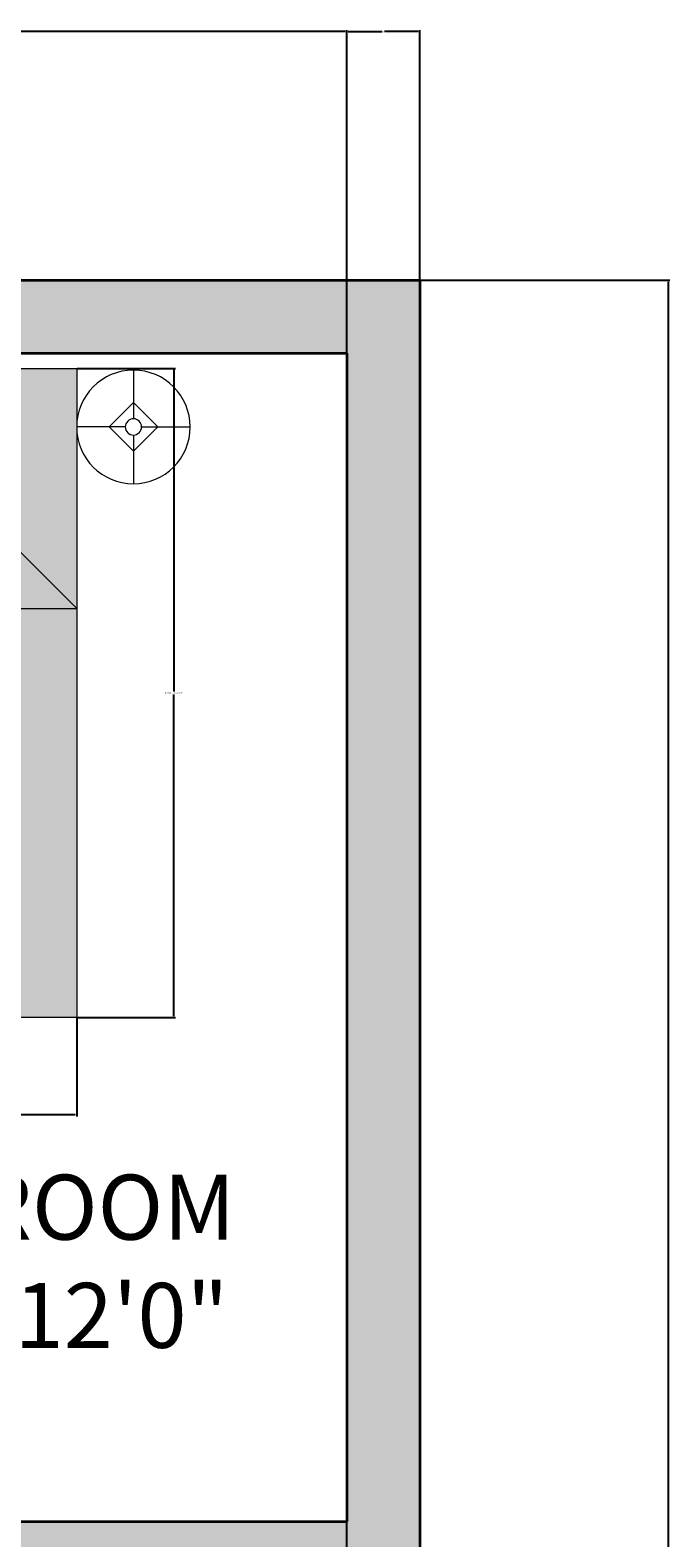
# Model space of a CAD drawing. Units: inches. Extents: x 1567 to 1964, y 1813 to 2447.
# Tile 28 of 28: x 1885 to 1964, y 2261 to 2447. Entities that reach past the tile are written whole.
import ezdxf

# ---------------------------------------------------------------- set-up
doc = ezdxf.new("R2010")
doc.units = ezdxf.units.IN
for name, color, linetype, lineweight in [('A-ANNO-DIMS', 2, 'Continuous', 18), ('A-AREA-IDEN', 7, 'Continuous', 18), ('A-FURN', 8, 'Continuous', 18), ('A-WALL', 7, 'Continuous', 35)]:
    doc.layers.add(name, color=color, linetype=linetype, lineweight=lineweight)
doc.layers.add('A-FURN-PATT', color=252, linetype='Continuous', lineweight=13, true_color=0x939598)
doc.layers.add('A-WALL-PATT', color=251, linetype='Continuous', lineweight=13, true_color=0x636466)
doc.styles.get("Standard").update_dxf_attribs({"font": 'arial.ttf'})
doc.dimstyles.get("Standard").update_dxf_attribs({"dimtxt": 0.18, "dimasz": 0.18, "dimexe": 0.18, "dimexo": 0.0625, "dimgap": 0.09, "dimtad": 0, "dimtih": 1, "dimtoh": 1, "dimdec": 4, "dimzin": 0, "dimdsep": 46, "dimtxsty": 'Standard', "dimcen": 0.09, "dimadec": 0, "dimazin": 0, "dimtfac": 1, "dimtdec": 4, "dimtofl": 0, "dimtmove": 0, "dimatfit": 3, "dimfxl": 1, "dimtolj": 1, "dimtzin": 0, "dimarcsym": 0})

# ---------------------------------------------------------------- blocks, each defined once
blk = doc.blocks.new('Bed - Queen')
for p, q in [((0, -80.00003), (0, 0)), ((0, 0), (59.99999, 0)), ((59.99999, 0), (59.99999, -80.00003)), ((7.99999, -1.2), (28.79998, -1.2)), ((7.99999, -14.4), (7.99999, -1.2)), ((28.79998, -1.2), (28.79998, -14.4)), ((31.19999, -1.2), (51.99999, -1.2)), ((31.19999, -14.4), (31.19999, -1.2)), ((51.99999, -1.2), (51.99999, -16.4)), ((0, -14.4), (44.8, -14.4)), ((59.99999, -29.6), (44.8, -14.4)), ((44.8, -14.4), (44.8, -29.6)), ((51.99999, -16.4), (46.79936, -16.4)), ((44.8, -16.8), (0, -16.8)), ((44.8, -29.6), (59.99999, -29.6)), ((59.99999, -80.00003), (0, -80.00003))]:
    blk.add_line(p, q)
blk = doc.blocks.new('Lamp - Table')
for p, q in [((0, 7), (0, 1)), ((0, 3), (-3, 0)), ((3, 0), (0, 3)), ((-1, 0), (-7, 0)), ((-3, 0), (0, -3)), ((0, -3), (3, 0)), ((1, 0), (7, 0)), ((0, -1), (0, -7))]:
    blk.add_line(p, q)
for radius in [7, 1]:
    blk.add_circle((0, 0), radius)
blk = doc.blocks.new('*D15')
at = {"layer": 'A-ANNO-DIMS', "color": 0, "lineweight": -2, "transparency": 16777216}
for p, q in [((1891.17, 2405.42), (1903.29, 2405.42)), ((1903.11, 2405.24), (1903.11, 2365.61)), ((1903.11, 2325.6), (1903.11, 2365.23)), ((1891.17, 2325.42), (1903.29, 2325.42))]:
    blk.add_line(p, q, dxfattribs=at)
at = {"layer": 'A-ANNO-DIMS', "color": 0, "transparency": 16777216}
for points in [[(1903.08, 2405.24), (1903.14, 2405.24), (1903.11, 2405.42)], [(1903.08, 2325.6), (1903.14, 2325.6), (1903.11, 2325.42)]]:
    blk.add_solid(points, dxfattribs=at)
at = {"layer": 'Defpoints', "color": 0, "transparency": 16777216}
for p in [(1891.11, 2405.42), (1903.11, 2405.42), (1891.11, 2325.42)]:
    blk.add_point(p, dxfattribs=at)
at = {"layer": 'A-ANNO-DIMS', "color": 0, "transparency": 16777216, "insert": (1903.11, 2365.42), "char_height": 0.18, "attachment_point": 5}
blk.add_mtext('\\A1;QUEEN BED 80 TYP.', dxfattribs=at)
blk = doc.blocks.new('*D16')
at = {"layer": 'A-ANNO-DIMS', "color": 0, "lineweight": -2, "transparency": 16777216}
for p, q in [((1831.11, 2325.36), (1831.11, 2313.24)), ((1891.11, 2325.36), (1891.11, 2313.24)), ((1831.29, 2313.42), (1860.58, 2313.42)), ((1890.93, 2313.42), (1861.64, 2313.42))]:
    blk.add_line(p, q, dxfattribs=at)
at = {"layer": 'A-ANNO-DIMS', "color": 0, "transparency": 16777216}
for points in [[(1831.29, 2313.45), (1831.29, 2313.39), (1831.11, 2313.42)], [(1890.93, 2313.45), (1890.93, 2313.39), (1891.11, 2313.42)]]:
    blk.add_solid(points, dxfattribs=at)
at = {"layer": 'Defpoints', "color": 0, "transparency": 16777216}
for p in [(1831.11, 2325.42), (1891.11, 2325.42), (1891.11, 2313.42)]:
    blk.add_point(p, dxfattribs=at)
at = {"layer": 'A-ANNO-DIMS', "color": 0, "transparency": 16777216, "insert": (1861.11, 2313.42), "char_height": 0.18, "attachment_point": 5}
blk.add_mtext('\\A1;60 TYP.', dxfattribs=at)
blk = doc.blocks.new('*D40')
at = {"layer": 'A-ANNO-DIMS', "color": 0, "lineweight": -2, "transparency": 16777216}
for p, q in [((1933.49, 2416.29), (1964.26, 2416.29)), ((1964.08, 2416.11), (1964.08, 2130.47)), ((1964.08, 1844.47), (1964.08, 2130.11)), ((1933.49, 1844.29), (1964.26, 1844.29))]:
    blk.add_line(p, q, dxfattribs=at)
at = {"layer": 'A-ANNO-DIMS', "color": 0, "transparency": 16777216}
for points in [[(1964.05, 2416.11), (1964.11, 2416.11), (1964.08, 2416.29)], [(1964.05, 1844.47), (1964.11, 1844.47), (1964.08, 1844.29)]]:
    blk.add_solid(points, dxfattribs=at)
at = {"layer": 'Defpoints', "color": 0, "transparency": 16777216}
for p in [(1933.43, 2416.29), (1964.08, 2416.29), (1933.43, 1844.29)]:
    blk.add_point(p, dxfattribs=at)
at = {"layer": 'A-ANNO-DIMS', "color": 0, "transparency": 16777216, "insert": (1964.08, 2130.29), "char_height": 0.18, "attachment_point": 5}
blk.add_mtext('\\A1;572', dxfattribs=at)
blk = doc.blocks.new('*D46')
at = {"layer": 'A-ANNO-DIMS', "color": 0, "lineweight": -2, "transparency": 16777216}
for p, q in [((1924.43, 2407.35), (1924.43, 2447.12)), ((1924.61, 2446.94), (1928.78, 2446.94)), ((1933.25, 2446.94), (1929.08, 2446.94)), ((1933.43, 2416.35), (1933.43, 2447.12))]:
    blk.add_line(p, q, dxfattribs=at)
at = {"layer": 'A-ANNO-DIMS', "color": 0, "transparency": 16777216}
for points in [[(1924.61, 2446.97), (1924.61, 2446.91), (1924.43, 2446.94)], [(1933.25, 2446.97), (1933.25, 2446.91), (1933.43, 2446.94)]]:
    blk.add_solid(points, dxfattribs=at)
at = {"layer": 'Defpoints', "color": 0, "transparency": 16777216}
for p in [(1924.43, 2446.94), (1933.43, 2416.29), (1924.43, 2407.29)]:
    blk.add_point(p, dxfattribs=at)
at = {"layer": 'A-ANNO-DIMS', "color": 0, "transparency": 16777216, "insert": (1928.93, 2446.94), "char_height": 0.18, "attachment_point": 5}
blk.add_mtext('\\A1;9', dxfattribs=at)
blk = doc.blocks.new('*D71')
at = {"layer": 'A-ANNO-DIMS', "color": 0, "lineweight": -2, "transparency": 16777216}
for p, q in [((1799.43, 1910.75), (1799.43, 2447.12)), ((1799.61, 2446.94), (1861.65, 2446.94)), ((1924.25, 2446.94), (1862.21, 2446.94)), ((1924.43, 1910.75), (1924.43, 2447.12))]:
    blk.add_line(p, q, dxfattribs=at)
at = {"layer": 'A-ANNO-DIMS', "color": 0, "transparency": 16777216}
for points in [[(1799.61, 2446.97), (1799.61, 2446.91), (1799.43, 2446.94)], [(1924.25, 2446.97), (1924.25, 2446.91), (1924.43, 2446.94)]]:
    blk.add_solid(points, dxfattribs=at)
at = {"layer": 'Defpoints', "color": 0, "transparency": 16777216}
for p in [(1924.43, 2446.94), (1799.43, 1910.69), (1924.43, 1910.69)]:
    blk.add_point(p, dxfattribs=at)
at = {"layer": 'A-ANNO-DIMS', "color": 0, "transparency": 16777216, "insert": (1861.93, 2446.94), "char_height": 0.18, "attachment_point": 5}
blk.add_mtext('\\A1;125', dxfattribs=at)

msp = doc.modelspace()

# ---------------------------------------------------------------- hatches: boundary and pattern name
at = {"layer": 'A-FURN-PATT'}
h = msp.add_hatch(color=256, dxfattribs=at)
h.dxf.hatch_style = 1
h.paths.add_polyline_path([(1621.2532, 2242.0229), (1643.7811, 2241.7239), (1643.8607, 2247.7234), (1617.863, 2248.0685, 0.19047621), (1616.7481, 2164.0759), (1642.7458, 2163.7308), (1642.8254, 2169.7302), (1620.2975, 2170.0293, -0.15194781)])
h.paths.add_polyline_path([(1673.5306, 2249.6607), (1653.8509, 2249.6607), (1653.8509, 2248.5031, 0.11764706), (1673.5306, 2248.5031)])
h.paths.add_polyline_path([(1706.0889, 2249.6607), (1686.4092, 2249.6607), (1686.4092, 2248.5031, 0.11764706), (1706.0889, 2248.5031)])
h.paths.add_polyline_path([(1782.4511, 2227.4197), (1766.4511, 2227.4197), (1766.2949, 2226.4197), (1782.6074, 2226.4197)])
h.paths.add_polyline_path([(1810.4511, 2227.4197), (1794.4511, 2227.4197), (1794.2949, 2226.4197), (1810.6074, 2226.4197)])
h.paths.add_polyline_path([(1743.9511, 2208.076), (1742.9511, 2207.9197), (1742.9511, 2191.9197), (1743.9511, 2191.7635)])
h.paths.add_polyline_path([(1782.6074, 2173.4197), (1766.2949, 2173.4197), (1766.4511, 2172.4197), (1782.4511, 2172.4197)])
h.paths.add_polyline_path([(1810.6074, 2173.4197), (1794.2949, 2173.4197), (1794.4511, 2172.4197), (1810.4511, 2172.4197)])
h.paths.add_polyline_path([(1861.053, 2006.5071), (1845.8531, 2006.5071), (1861.053, 1991.3071)])
h.paths.add_polyline_path([(1905.853, 1993.7071), (1861.053, 1993.7071), (1861.053, 1991.3071), (1905.853, 1991.3071)])
h.paths.add_polyline_path([(1919.7245, 2257.29, 0.50000012), (1918.7245, 2258.29), (1901.7245, 2258.29, 0.50000012), (1900.7245, 2257.29), (1900.7245, 2253.29, 0.50000012), (1901.7245, 2252.29), (1918.7245, 2252.29, 0.50000012), (1919.7245, 2253.29)])
h.paths.add_polyline_path([(1875.9094, 2391.0204), (1875.9094, 2375.8204), (1891.1093, 2375.8204)], flags=17)
h.paths.add_polyline_path([(1891.1093, 2405.4204), (1831.1094, 2405.4204), (1831.1094, 2391.0204), (1839.1093, 2391.0204), (1839.1093, 2404.2204), (1859.9093, 2404.2204), (1859.9093, 2391.0204), (1862.3093, 2391.0204), (1862.3093, 2404.2204), (1883.1093, 2404.2204), (1883.1093, 2389.0204), (1877.9094, 2389.0204), (1891.1093, 2375.8204)])
h.paths.add_polyline_path([(1682.1402, 2390.0316), (1682.1402, 2374.8316), (1697.3402, 2374.8316)], flags=17)
h.paths.add_polyline_path([(1697.3402, 2404.4316), (1637.3402, 2404.4316), (1637.3402, 2390.0316), (1645.3402, 2390.0316), (1645.3402, 2403.2316), (1666.1402, 2403.2316), (1666.1402, 2390.0316), (1668.5402, 2390.0316), (1668.5402, 2403.2316), (1689.3402, 2403.2316), (1689.3402, 2388.0316), (1684.1402, 2388.0316), (1697.3402, 2374.8316)])
h = msp.add_hatch(color=256, dxfattribs=at)
h.dxf.hatch_style = 1
h.paths.add_polyline_path([(1697.3402, 2374.8316), (1682.1402, 2374.8316), (1682.1402, 2387.6316), (1637.3402, 2387.6316), (1637.3402, 2324.4315), (1697.3402, 2324.4315)])
h.paths.add_polyline_path([(1891.1093, 2375.8204), (1875.9094, 2375.8204), (1875.9094, 2388.6204), (1831.1094, 2388.6204), (1831.1094, 2325.4204), (1891.1093, 2325.4204)])
h.paths.add_polyline_path([(1702.5611, 2206.8057), (1702.5611, 2210.8057), (1699.7395, 2209.9436), (1697.013, 2209.2403), (1694.3857, 2208.6763), (1691.8615, 2208.2326), (1689.4443, 2207.8896), (1687.1381, 2207.6282), (1684.9469, 2207.4289), (1682.8747, 2207.2725), (1680.9233, 2207.1425), (1679.0865, 2207.0339), (1677.3558, 2206.9445), (1675.7229, 2206.8719), (1674.1794, 2206.8141), (1672.7169, 2206.7688), (1671.327, 2206.7339), (1670.0014, 2206.707), (1668.7314, 2206.6866), (1667.5072, 2206.6732), (1666.3188, 2206.668), (1665.1561, 2206.6722), (1664.009, 2206.6869), (1662.8675, 2206.7133), (1661.7215, 2206.7525), (1660.5611, 2206.8057), (1660.5611, 2202.8057), (1661.9932, 2202.9556), (1663.3314, 2203.0744), (1664.5899, 2203.1671), (1665.7831, 2203.2385), (1666.9254, 2203.2935), (1668.0311, 2203.3368), (1669.1145, 2203.3734), (1670.1902, 2203.4081), (1671.2724, 2203.4451), (1672.3759, 2203.4866), (1673.5155, 2203.534), (1674.706, 2203.5887), (1675.9621, 2203.6523), (1677.2986, 2203.7262), (1678.7304, 2203.8118), (1680.2722, 2203.9108), (1681.947, 2204.0272), (1683.8108, 2204.1769), (1685.9279, 2204.3782), (1688.3626, 2204.6496), (1691.179, 2205.0096), (1694.4413, 2205.4767), (1698.214, 2206.0692)])
h.paths.add_polyline_path([(1702.5611, 2218.8057), (1701.9821, 2217.9383), (1701.3316, 2217.191), (1700.6091, 2216.5515), (1699.8141, 2216.0071), (1698.946, 2215.5454), (1698.0041, 2215.1536), (1696.9879, 2214.8194), (1695.8969, 2214.5301), (1694.7328, 2214.2753), (1693.5072, 2214.0522), (1692.2339, 2213.8602), (1690.9266, 2213.6989), (1689.5994, 2213.5675), (1688.266, 2213.4654), (1686.9402, 2213.392), (1685.636, 2213.3467), (1684.3619, 2213.3287), (1683.1053, 2213.3361), (1681.8482, 2213.3668), (1680.5727, 2213.4187), (1679.2608, 2213.4898), (1677.8948, 2213.5779), (1676.4565, 2213.6811), (1674.9282, 2213.7971), (1673.2982, 2213.9236), (1671.5804, 2214.0573), (1669.795, 2214.1945), (1667.9622, 2214.3316), (1666.1022, 2214.4649), (1664.2352, 2214.5908), (1662.3814, 2214.7056), (1660.5611, 2214.8057), (1660.5611, 2206.8057), (1661.7215, 2206.7525), (1662.8675, 2206.7133), (1664.009, 2206.6869), (1665.1561, 2206.6722), (1666.3188, 2206.668), (1667.5072, 2206.6732), (1668.7314, 2206.6866), (1670.0014, 2206.707), (1671.327, 2206.7339), (1672.7169, 2206.7688), (1674.1794, 2206.8141), (1675.7229, 2206.8719), (1677.3558, 2206.9445), (1679.0865, 2207.0339), (1680.9233, 2207.1425), (1682.8747, 2207.2725), (1684.9469, 2207.4289), (1687.1381, 2207.6282), (1689.4443, 2207.8896), (1691.8615, 2208.2326), (1694.3857, 2208.6763), (1697.013, 2209.2403), (1699.7395, 2209.9436), (1702.5611, 2210.8057)])
h.paths.add_polyline_path([(1700.6091, 2216.5515), (1701.3316, 2217.191), (1701.9821, 2217.9383), (1702.5611, 2218.8057), (1702.5611, 2222.8057), (1689.452, 2222.8057), (1689.0171, 2222.4556), (1688.4521, 2222.0354), (1687.7806, 2221.5662), (1687.0235, 2221.067), (1686.2019, 2220.5566), (1685.3367, 2220.0541), (1684.4491, 2219.5785), (1683.56, 2219.1486), (1682.6867, 2218.7795), (1681.8312, 2218.4692), (1680.9918, 2218.212), (1680.1667, 2218.0019), (1679.3541, 2217.833), (1678.5524, 2217.6995), (1677.7597, 2217.5954), (1676.9744, 2217.5149), (1676.1942, 2217.4531), (1675.4146, 2217.4093), (1674.6309, 2217.384), (1673.8381, 2217.3774), (1673.0313, 2217.39), (1672.2056, 2217.4221), (1671.3562, 2217.4741), (1670.4782, 2217.5463), (1669.5642, 2217.639), (1668.5968, 2217.7516), (1667.5562, 2217.8833), (1666.4226, 2218.0336), (1665.1761, 2218.2017), (1663.7969, 2218.3869), (1662.2651, 2218.5885), (1660.5611, 2218.8057), (1660.5611, 2214.8057), (1662.3814, 2214.7056), (1664.2352, 2214.5908), (1666.1022, 2214.4649), (1667.9622, 2214.3316), (1669.795, 2214.1945), (1671.5804, 2214.0573), (1673.2982, 2213.9236), (1674.9282, 2213.7971), (1676.4565, 2213.6811), (1677.8948, 2213.5779), (1679.2608, 2213.4898), (1680.5727, 2213.4187), (1681.8482, 2213.3668), (1683.1053, 2213.3361), (1684.3619, 2213.3287), (1685.636, 2213.3467), (1686.9402, 2213.392), (1688.266, 2213.4654), (1689.5994, 2213.5675), (1690.9266, 2213.6989), (1692.2339, 2213.8602), (1693.5072, 2214.0522), (1694.7328, 2214.2753), (1695.8969, 2214.5301), (1696.9879, 2214.8194), (1698.0041, 2215.1536), (1698.946, 2215.5454), (1699.8141, 2216.0071)])
h.paths.add_polyline_path([(1687.0235, 2221.067), (1687.7806, 2221.5662), (1688.4521, 2222.0354), (1689.0171, 2222.4556), (1689.452, 2222.8057), (1660.5611, 2222.8057), (1660.5611, 2218.8057), (1662.2651, 2218.5885), (1663.7969, 2218.3869), (1665.1761, 2218.2017), (1666.4226, 2218.0336), (1667.5562, 2217.8833), (1668.5968, 2217.7516), (1669.5642, 2217.639), (1670.4782, 2217.5463), (1671.3562, 2217.4741), (1672.2056, 2217.4221), (1673.0313, 2217.39), (1673.8381, 2217.3774), (1674.6309, 2217.384), (1675.4146, 2217.4093), (1676.1942, 2217.4531), (1676.9744, 2217.5149), (1677.7597, 2217.5954), (1678.5524, 2217.6995), (1679.3541, 2217.833), (1680.1667, 2218.0019), (1680.9918, 2218.212), (1681.8312, 2218.4692), (1682.6867, 2218.7795), (1683.56, 2219.1486), (1684.4491, 2219.5785), (1685.3367, 2220.0541), (1686.2019, 2220.5566)], flags=17)
h.paths.add_polyline_path([(1702.5611, 2198.8057), (1698.9289, 2199.2412), (1695.8472, 2199.5774), (1693.2166, 2199.8257), (1690.9377, 2199.9973), (1688.9111, 2200.1033), (1687.0375, 2200.155), (1685.2174, 2200.1637), (1683.3514, 2200.1406), (1681.3514, 2200.0941), (1679.1736, 2200.0225), (1676.7858, 2199.921), (1674.1554, 2199.7852), (1671.2502, 2199.6103), (1668.0377, 2199.3919), (1664.4854, 2199.1252), (1660.5611, 2198.8057), (1660.5611, 2194.8057), (1662.2697, 2194.9771), (1663.9673, 2195.0999), (1665.6339, 2195.1809), (1667.2495, 2195.227), (1668.7941, 2195.2449), (1670.2478, 2195.2414), (1671.5906, 2195.2233), (1672.8026, 2195.1974), (1673.8739, 2195.1689), (1674.8359, 2195.1364), (1675.7302, 2195.0967), (1676.5982, 2195.0469), (1677.4817, 2194.9838), (1678.422, 2194.9043), (1679.4609, 2194.8055), (1680.6397, 2194.6842), (1682.005, 2194.5341), (1683.6223, 2194.335), (1685.562, 2194.0637), (1687.8945, 2193.6967), (1690.6902, 2193.2108), (1694.0196, 2192.5826), (1697.9531, 2191.7887), (1702.5611, 2190.8057)])
h.paths.add_polyline_path([(1702.5611, 2206.8057), (1698.214, 2206.0692), (1694.4413, 2205.4767), (1691.179, 2205.0096), (1688.3626, 2204.6496), (1685.9279, 2204.3782), (1683.8108, 2204.1769), (1681.947, 2204.0272), (1680.2722, 2203.9108), (1678.7304, 2203.8118), (1677.2986, 2203.7262), (1675.9621, 2203.6523), (1674.706, 2203.5887), (1673.5155, 2203.534), (1672.3759, 2203.4866), (1671.2724, 2203.4451), (1670.1902, 2203.4081), (1669.1145, 2203.3734), (1668.0311, 2203.3368), (1666.9254, 2203.2935), (1665.7831, 2203.2385), (1664.5899, 2203.1671), (1663.3314, 2203.0744), (1661.9932, 2202.9556), (1660.5611, 2202.8057), (1660.5611, 2198.8057), (1664.4854, 2199.1252), (1668.0377, 2199.3919), (1671.2502, 2199.6103), (1674.1554, 2199.7852), (1676.7858, 2199.921), (1679.1736, 2200.0225), (1681.3514, 2200.0941), (1683.3514, 2200.1406), (1685.2174, 2200.1637), (1687.0375, 2200.155), (1688.9111, 2200.1033), (1690.9377, 2199.9973), (1693.2166, 2199.8257), (1695.8472, 2199.5774), (1698.9289, 2199.2412), (1702.5611, 2198.8057)])
h.paths.add_polyline_path([(1702.5611, 2190.8057), (1697.9531, 2191.7887), (1694.0196, 2192.5826), (1690.6902, 2193.2108), (1687.8945, 2193.6967), (1685.562, 2194.0637), (1683.6223, 2194.335), (1682.005, 2194.5341), (1680.6397, 2194.6842), (1679.4609, 2194.8055), (1678.422, 2194.9043), (1677.4817, 2194.9838), (1676.5982, 2195.0469), (1675.7302, 2195.0967), (1674.8359, 2195.1364), (1673.8739, 2195.1689), (1672.8026, 2195.1974), (1671.5906, 2195.2233), (1670.2478, 2195.2414), (1668.7941, 2195.2449), (1667.2495, 2195.227), (1665.6339, 2195.1809), (1663.9673, 2195.0999), (1662.2697, 2194.9771), (1660.5611, 2194.8057), (1660.5611, 2190.8057), (1665.9637, 2190.2699), (1670.5105, 2189.7867), (1674.3035, 2189.3504), (1677.4445, 2188.9552), (1680.0354, 2188.5951), (1682.1782, 2188.2644), (1683.9747, 2187.9571), (1685.5268, 2187.6675), (1686.9225, 2187.3901), (1688.1943, 2187.1216), (1689.3606, 2186.859), (1690.4399, 2186.5993), (1691.4508, 2186.3396), (1692.4118, 2186.0769), (1693.3413, 2185.8084), (1694.2579, 2185.531), (1695.1786, 2185.2422), (1696.1142, 2184.9406), (1697.0739, 2184.6252), (1698.0671, 2184.2949), (1699.1032, 2183.9489), (1700.1913, 2183.586), (1701.3408, 2183.2053), (1702.5611, 2182.8057)])
h.paths.add_polyline_path([(1702.5611, 2182.8057), (1701.3408, 2183.2053), (1700.1913, 2183.586), (1699.1032, 2183.9489), (1698.0671, 2184.2949), (1697.0739, 2184.6252), (1696.1142, 2184.9406), (1695.1786, 2185.2422), (1694.2579, 2185.531), (1693.3413, 2185.8084), (1692.4118, 2186.0769), (1691.4508, 2186.3396), (1690.4399, 2186.5993), (1689.3606, 2186.859), (1688.1943, 2187.1216), (1686.9225, 2187.3901), (1685.5268, 2187.6675), (1683.9747, 2187.9571), (1682.1782, 2188.2644), (1680.0354, 2188.5951), (1677.4445, 2188.9552), (1674.3035, 2189.3504), (1670.5105, 2189.7867), (1665.9637, 2190.2699), (1660.5611, 2190.8057), (1660.5611, 2186.8057), (1663.5709, 2186.52), (1666.0965, 2186.2414), (1668.1979, 2185.9698), (1669.9351, 2185.7048), (1671.3681, 2185.446), (1672.5568, 2185.1931), (1673.5613, 2184.9458), (1674.4415, 2184.7037), (1675.2485, 2184.4664), (1675.9976, 2184.2328), (1677.0295, 2183.8907), (1678.2492, 2183.4332), (1679.354, 2182.9669), (1680.4123, 2182.4724), (1681.3757, 2181.9718), (1682.2435, 2181.4594), (1683.1864, 2180.8057), (1702.5611, 2180.8057)])
h.paths.add_polyline_path([(1677.3469, 2183.7716), (1676.6949, 2184.0016), (1675.9976, 2184.2328), (1675.2485, 2184.4664), (1674.4415, 2184.7037), (1673.5613, 2184.9458), (1672.5568, 2185.1931), (1671.3681, 2185.446), (1669.9351, 2185.7048), (1668.1979, 2185.9698), (1666.0965, 2186.2414), (1663.5709, 2186.52), (1660.5611, 2186.8057), (1660.5611, 2180.8057), (1683.1506, 2180.8057), (1682.802, 2181.0722), (1682.4264, 2181.3326), (1682.0201, 2181.5913), (1681.586, 2181.8476), (1681.1268, 2182.1011), (1680.6453, 2182.3513), (1680.1443, 2182.5976), (1679.6266, 2182.8395), (1679.0933, 2183.0769), (1678.5398, 2183.3105), (1677.9598, 2183.5417)], flags=17)
h.paths.add_polyline_path([(1824.4511, 2199.9016), (1824.089, 2199.9302), (1824.0595, 2199.9372), (1824.0397, 2199.9406), (1823.5413, 2200.0576), (1823.4095, 2200.0864), (1823.0664, 2200.1559), (1822.6419, 2200.2361), (1822.1519, 2200.3222), (1821.6126, 2200.4093), (1821.0401, 2200.4925), (1820.4505, 2200.5669), (1819.8599, 2200.6276), (1819.2845, 2200.6697), (1818.7366, 2200.6896), (1818.2141, 2200.688), (1817.7112, 2200.6668), (1817.222, 2200.6281), (1816.7405, 2200.5737), (1816.261, 2200.5057), (1815.7776, 2200.4259), (1815.2845, 2200.3364), (1814.3007, 2200.149), (1813.3315, 2199.9765), (1812.406, 2199.8514), (1811.6868, 2199.7739), (1810.8992, 2199.7121), (1810.0345, 2199.6697), (1809.0854, 2199.6497), (1808.0514, 2199.6502), (1806.9334, 2199.6683), (1805.7324, 2199.701), (1804.4493, 2199.7454), (1803.0852, 2199.7986), (1801.641, 2199.8577), (1800.1178, 2199.9197), (1798.5134, 2199.9818), (1796.8144, 2200.0415), (1795.004, 2200.0962), (1793.0657, 2200.1437), (1790.9828, 2200.1814), (1788.7389, 2200.2068), (1786.3171, 2200.2177), (1783.7011, 2200.2114), (1780.8715, 2200.185), (1777.7988, 2200.1326), (1774.4506, 2200.0481), (1770.7948, 2199.9249), (1766.7992, 2199.7569), (1762.4316, 2199.5376), (1757.6596, 2199.2606), (1752.4511, 2198.9197), (1752.4511, 2193.4197), (1761.2668, 2193.6071), (1768.3671, 2193.7934), (1773.9821, 2193.9778), (1778.3417, 2194.1593), (1781.6759, 2194.3369), (1784.2148, 2194.5096), (1786.1882, 2194.6764), (1787.8261, 2194.8364), (1789.3219, 2194.9887), (1790.7226, 2195.1333), (1792.0383, 2195.27), (1793.2792, 2195.3989), (1794.4557, 2195.52), (1795.5781, 2195.6333), (1796.6564, 2195.7387), (1797.7011, 2195.8364), (1798.7216, 2195.9259), (1799.7245, 2196.0057), (1800.7158, 2196.0737), (1801.7011, 2196.1281), (1802.6865, 2196.1668), (1803.6777, 2196.188), (1804.6806, 2196.1896), (1805.7011, 2196.1697), (1806.7423, 2196.1273), (1807.7962, 2196.0643), (1808.852, 2195.9837), (1809.899, 2195.8885), (1810.9265, 2195.7815), (1811.9238, 2195.6658), (1812.88, 2195.5442), (1813.7845, 2195.4197), (1814.6296, 2195.2948), (1815.4205, 2195.1704), (1816.1656, 2195.0469), (1816.873, 2194.9249), (1817.5511, 2194.8049), (1818.2083, 2194.6873), (1818.8527, 2194.5726), (1819.4928, 2194.4614), (1820.1348, 2194.3554), (1820.7773, 2194.2615), (1821.4169, 2194.1882), (1822.0501, 2194.1437), (1822.6735, 2194.1363), (1823.2838, 2194.1743), (1823.8775, 2194.266), (1824.4511, 2194.4197)])
h.paths.add_polyline_path([(1821.4716, 2190.5098), (1820.4303, 2190.5708), (1819.3811, 2190.6415), (1818.3339, 2190.7186), (1817.2985, 2190.7986), (1816.2845, 2190.8781), (1815.2976, 2190.9542), (1814.3274, 2191.0259), (1813.3592, 2191.0927), (1812.3782, 2191.1541), (1811.3699, 2191.2097), (1810.3196, 2191.2589), (1809.2127, 2191.3013), (1808.0345, 2191.3364), (1806.7708, 2191.3634), (1805.4094, 2191.3807), (1803.9387, 2191.3862), (1802.3469, 2191.3781), (1800.6223, 2191.3543), (1798.7532, 2191.313), (1796.7278, 2191.2521), (1794.5344, 2191.1697), (1792.128, 2191.0648), (1789.33, 2190.9393), (1785.9285, 2190.7962), (1781.7115, 2190.6385), (1776.4672, 2190.469), (1769.9836, 2190.2908), (1762.0489, 2190.1067), (1752.4511, 2189.9197), (1752.4511, 2185.4197), (1758.363, 2185.5846), (1763.4179, 2185.7075), (1767.7199, 2185.7933), (1771.373, 2185.8468), (1774.4811, 2185.873), (1777.1484, 2185.8768), (1779.4787, 2185.8629), (1781.5761, 2185.8364), (1783.5287, 2185.8014), (1785.3606, 2185.7596), (1787.0802, 2185.7119), (1788.6959, 2185.6593), (1790.2158, 2185.6028), (1791.6484, 2185.5434), (1793.0018, 2185.4821), (1794.2844, 2185.4197), (1795.5065, 2185.3576), (1796.6861, 2185.298), (1797.8433, 2185.2432), (1798.998, 2185.1958), (1800.1703, 2185.1581), (1801.3801, 2185.1326), (1802.6476, 2185.1218), (1803.9928, 2185.1281), (1805.4444, 2185.1555), (1807.0663, 2185.2147), (1808.9315, 2185.3178), (1811.1126, 2185.477), (1813.6823, 2185.7046), (1816.7135, 2186.0128), (1820.2788, 2186.4138), (1824.4511, 2186.9197), (1824.4511, 2190.4197), (1823.4918, 2190.4309), (1822.4954, 2190.4621)])
h.paths.add_polyline_path([(1797.3762, 2216.0584), (1797.6199, 2216.2267), (1797.9558, 2216.3355), (1798.3017, 2216.3703), (1798.5761, 2216.3781), (1798.8974, 2216.3703), (1799.2714, 2216.3468), (1799.704, 2216.3078), (1800.2011, 2216.2531), (1800.7695, 2216.1829), (1801.4205, 2216.0981), (1802.1662, 2215.9996), (1803.0188, 2215.8885), (1803.9906, 2215.7656), (1805.0937, 2215.632), (1806.3404, 2215.4886), (1807.7428, 2215.3364), (1809.3101, 2215.1764), (1811.039, 2215.0096), (1812.9232, 2214.8369), (1814.9563, 2214.6593), (1817.132, 2214.4778), (1819.444, 2214.2934), (1821.8858, 2214.1071), (1824.4511, 2213.9197), (1824.4511, 2217.9197), (1752.4511, 2217.9197), (1752.4511, 2214.9197), (1757.2739, 2214.8973), (1761.6432, 2214.8338), (1765.5973, 2214.7352), (1769.1751, 2214.6072), (1772.4149, 2214.4559), (1775.3554, 2214.2869), (1778.0352, 2214.1063), (1780.4928, 2213.9197), (1782.7607, 2213.7329), (1784.8476, 2213.5499), (1786.7557, 2213.3748), (1788.4876, 2213.2114), (1790.0456, 2213.0636), (1791.4322, 2212.9354), (1792.6499, 2212.8305), (1793.7011, 2212.7531), (1794.5904, 2212.7059), (1795.3313, 2212.688), (1795.9394, 2212.6974), (1796.4303, 2212.7322), (1796.8196, 2212.7905), (1797.123, 2212.8703), (1797.356, 2212.9695), (1797.5344, 2213.0864), (1797.6716, 2213.2187), (1797.7727, 2213.3637), (1797.8406, 2213.5185), (1797.8782, 2213.6801), (1797.8884, 2213.8457), (1797.8743, 2214.0122), (1797.8386, 2214.1767), (1797.7844, 2214.3364), (1797.7149, 2214.4889), (1797.6347, 2214.6346), (1797.5486, 2214.7744), (1797.3327, 2215.109), (1797.178, 2215.4303), (1797.1896, 2215.7939)])
h.paths.add_polyline_path([(1804.7872, 2210.6789), (1804.546, 2211.022), (1804.3512, 2211.3917), (1804.2466, 2211.7546), (1804.2574, 2212.0998), (1804.4058, 2212.4178), (1804.7068, 2212.7007), (1805.1359, 2212.9124), (1805.5279, 2212.9926), (1805.8136, 2213.0154), (1806.1178, 2213.0031), (1806.4405, 2212.9529), (1806.7929, 2212.867), (1807.1893, 2212.7489), (1807.6438, 2212.602), (1808.1706, 2212.4297), (1808.7838, 2212.2355), (1809.4976, 2212.0227), (1810.3261, 2211.7947), (1811.2868, 2211.5533), (1812.4101, 2211.2928), (1813.7297, 2211.0059), (1815.2793, 2210.6854), (1817.0925, 2210.3238), (1819.2031, 2209.9139), (1821.6447, 2209.4483), (1824.4511, 2208.9197), (1824.4511, 2213.9197), (1821.8858, 2214.1071), (1819.444, 2214.2934), (1817.132, 2214.4778), (1814.9563, 2214.6593), (1812.9232, 2214.8369), (1811.039, 2215.0096), (1809.3101, 2215.1764), (1807.7428, 2215.3364), (1806.3404, 2215.4886), (1805.0937, 2215.632), (1803.9906, 2215.7656), (1803.0188, 2215.8885), (1802.1662, 2215.9996), (1801.4205, 2216.0981), (1800.7695, 2216.1829), (1800.2011, 2216.2531), (1799.704, 2216.3078), (1799.2714, 2216.3468), (1798.8974, 2216.3703), (1798.5761, 2216.3781), (1798.3017, 2216.3703), (1798.0683, 2216.3468), (1797.87, 2216.3078), (1797.7011, 2216.2531), (1797.5566, 2216.1831), (1797.4355, 2216.0994), (1797.3378, 2216.004), (1797.2636, 2215.8989), (1797.2128, 2215.7859), (1797.1855, 2215.6671), (1797.1816, 2215.5444), (1797.2011, 2215.4197), (1797.2433, 2215.2946), (1797.304, 2215.1684), (1797.3783, 2215.0403), (1797.4615, 2214.9093), (1797.6718, 2214.5836), (1797.8218, 2214.2545), (1797.8933, 2213.9247), (1797.8728, 2213.5918), (1797.7366, 2213.2814), (1797.4586, 2213.0132), (1797.123, 2212.8703), (1796.8196, 2212.7905), (1796.4303, 2212.7322), (1795.9394, 2212.6974), (1795.3313, 2212.688), (1794.5904, 2212.7059), (1793.7011, 2212.7531), (1792.6499, 2212.8305), (1791.4322, 2212.9354), (1790.0456, 2213.0636), (1788.4876, 2213.2114), (1786.7557, 2213.3748), (1784.8476, 2213.5499), (1782.7607, 2213.7329), (1780.4928, 2213.9197), (1778.0352, 2214.1063), (1775.3554, 2214.2869), (1772.4149, 2214.4559), (1769.1751, 2214.6072), (1765.5973, 2214.7352), (1761.6432, 2214.8338), (1757.2739, 2214.8973), (1752.4511, 2214.9197), (1752.4511, 2209.9197), (1759.4745, 2210.0625), (1765.2786, 2210.1242), (1770.027, 2210.1175), (1773.8834, 2210.0551), (1777.0112, 2209.9498), (1779.5741, 2209.8143), (1781.7357, 2209.6611), (1783.6594, 2209.5031), (1785.4813, 2209.3506), (1787.2265, 2209.2049), (1788.8926, 2209.0651), (1790.4771, 2208.9301), (1791.9777, 2208.7991), (1793.3919, 2208.671), (1794.7171, 2208.5449), (1795.9511, 2208.4197), (1797.0922, 2208.2952), (1798.1425, 2208.1736), (1799.1049, 2208.0579), (1799.9823, 2207.951), (1800.7778, 2207.8558), (1801.4941, 2207.7752), (1802.1342, 2207.7122), (1802.7011, 2207.6697), (1803.1982, 2207.65), (1803.6308, 2207.6528), (1804.0048, 2207.6771), (1804.3261, 2207.7218), (1804.6005, 2207.7861), (1804.8339, 2207.869), (1805.0322, 2207.9694), (1805.2011, 2208.0864), (1805.3455, 2208.2189), (1805.4654, 2208.365), (1805.56, 2208.5229), (1805.6282, 2208.6906), (1805.6691, 2208.866), (1805.6816, 2209.0473), (1805.6648, 2209.2326), (1805.6178, 2209.4197), (1805.5406, 2209.6072), (1805.4381, 2209.7947), (1805.316, 2209.9822), (1805.1803, 2210.1697), (1805.0367, 2210.3572)])
h.paths.add_polyline_path([(1801.4941, 2207.7752), (1800.7778, 2207.8558), (1799.9823, 2207.951), (1799.1049, 2208.0579), (1798.1425, 2208.1736), (1797.0922, 2208.2952), (1795.9511, 2208.4197), (1794.7171, 2208.5449), (1793.3919, 2208.671), (1791.9777, 2208.7991), (1790.4771, 2208.9301), (1788.8926, 2209.0651), (1787.2265, 2209.2049), (1785.4813, 2209.3506), (1783.6594, 2209.5031), (1781.7357, 2209.6611), (1779.5741, 2209.8143), (1777.0112, 2209.9498), (1773.8834, 2210.0551), (1770.027, 2210.1175), (1765.2786, 2210.1242), (1759.4745, 2210.0625), (1752.4511, 2209.9197), (1752.4511, 2205.4197), (1757.7354, 2205.2545), (1762.3821, 2205.1294), (1766.4565, 2205.0374), (1770.024, 2204.9718), (1773.1502, 2204.9258), (1775.9003, 2204.8924), (1778.3399, 2204.8649), (1780.5344, 2204.8364), (1782.5421, 2204.8014), (1784.3925, 2204.7596), (1786.1082, 2204.7119), (1787.7115, 2204.6593), (1789.225, 2204.6028), (1790.6711, 2204.5434), (1792.0724, 2204.4821), (1793.4511, 2204.4197), (1794.8241, 2204.3576), (1796.1855, 2204.2973), (1797.5234, 2204.241), (1798.8261, 2204.1906), (1800.082, 2204.1479), (1801.2792, 2204.115), (1802.4062, 2204.0939), (1803.4511, 2204.0864), (1804.4051, 2204.0942), (1805.2701, 2204.1176), (1806.0512, 2204.1567), (1806.7532, 2204.2114), (1807.381, 2204.2817), (1807.9394, 2204.3676), (1808.4334, 2204.4692), (1808.8678, 2204.5864), (1809.248, 2204.7187), (1809.5813, 2204.8637), (1809.8756, 2205.0185), (1810.1386, 2205.1801), (1810.3782, 2205.3457), (1810.6022, 2205.5122), (1810.9725, 2205.7941), (1811.3803, 2206.072), (1811.739, 2206.2612), (1812.0032, 2206.3781), (1812.2869, 2206.4793), (1812.5931, 2206.563), (1812.9246, 2206.6271), (1813.2845, 2206.6697), (1813.6746, 2206.6894), (1814.0931, 2206.6867), (1814.5369, 2206.6624), (1815.0032, 2206.6176), (1815.489, 2206.5534), (1815.9915, 2206.4705), (1816.5076, 2206.3701), (1817.0345, 2206.2531), (1817.5753, 2206.1196), (1818.1582, 2205.9666), (1818.8172, 2205.7902), (1819.5865, 2205.5864), (1820.5004, 2205.3514), (1821.5931, 2205.0812), (1822.8986, 2204.7719), (1824.4511, 2204.4197), (1824.4511, 2208.9197), (1821.6447, 2209.4483), (1819.2031, 2209.9139), (1817.0925, 2210.3238), (1815.2793, 2210.6854), (1813.7297, 2211.0059), (1812.4101, 2211.2928), (1811.2868, 2211.5533), (1810.3261, 2211.7947), (1809.4976, 2212.0227), (1808.7838, 2212.2355), (1808.1706, 2212.4297), (1807.6438, 2212.602), (1807.1893, 2212.7489), (1806.7929, 2212.867), (1806.4405, 2212.9529), (1806.1178, 2213.0031), (1805.8136, 2213.0154), (1805.5279, 2212.9926), (1805.2638, 2212.9386), (1805.024, 2212.8572), (1804.8116, 2212.7524), (1804.6295, 2212.6281), (1804.4806, 2212.4881), (1804.3678, 2212.3364), (1804.2931, 2212.1764), (1804.2545, 2212.0096), (1804.2491, 2211.8369), (1804.274, 2211.6593), (1804.3263, 2211.4778), (1804.4029, 2211.2934), (1804.5011, 2211.1071), (1804.6178, 2210.9197), (1804.7496, 2210.7322), (1804.8912, 2210.5447), (1805.154, 2210.2061), (1805.3962, 2209.8715), (1805.5964, 2209.5053), (1805.688, 2209.1402), (1805.6629, 2208.7758), (1805.5257, 2208.4385), (1805.2839, 2208.1437), (1804.9434, 2207.9078), (1804.6005, 2207.7861), (1804.3261, 2207.7218), (1804.0048, 2207.6771), (1803.6308, 2207.6528), (1803.1982, 2207.65), (1802.7011, 2207.6697), (1802.1342, 2207.7122)])
h.paths.add_polyline_path([(1824.4511, 2204.4197), (1822.8986, 2204.7719), (1821.5931, 2205.0812), (1820.5004, 2205.3514), (1819.5865, 2205.5864), (1818.8172, 2205.7902), (1818.1582, 2205.9666), (1817.5753, 2206.1196), (1817.0345, 2206.2531), (1816.5076, 2206.3701), (1815.9915, 2206.4705), (1815.489, 2206.5534), (1815.0032, 2206.6176), (1814.5369, 2206.6624), (1814.0931, 2206.6867), (1813.6746, 2206.6894), (1813.2845, 2206.6697), (1812.9246, 2206.6271), (1812.5931, 2206.563), (1812.2869, 2206.4793), (1812.0032, 2206.3781), (1811.739, 2206.2612), (1811.4915, 2206.1307), (1811.2576, 2205.9884), (1811.0345, 2205.8364), (1810.8183, 2205.6767), (1810.4357, 2205.3854), (1810.1386, 2205.1801), (1809.8756, 2205.0185), (1809.5813, 2204.8637), (1809.248, 2204.7187), (1808.8678, 2204.5864), (1808.4334, 2204.4692), (1807.9394, 2204.3676), (1807.381, 2204.2817), (1806.7532, 2204.2114), (1806.0512, 2204.1567), (1805.2701, 2204.1176), (1804.4051, 2204.0942), (1803.4511, 2204.0864), (1802.4062, 2204.0939), (1801.2792, 2204.115), (1800.082, 2204.1479), (1798.8261, 2204.1906), (1797.5234, 2204.241), (1796.1855, 2204.2973), (1794.8241, 2204.3576), (1793.4511, 2204.4197), (1792.0724, 2204.4821), (1790.6711, 2204.5434), (1789.225, 2204.6028), (1787.7115, 2204.6593), (1786.1082, 2204.7119), (1784.3925, 2204.7596), (1782.5421, 2204.8014), (1780.5344, 2204.8364), (1778.3399, 2204.8649), (1775.9003, 2204.8924), (1773.1502, 2204.9258), (1770.024, 2204.9718), (1766.4565, 2205.0374), (1762.3821, 2205.1294), (1757.7354, 2205.2545), (1752.4511, 2205.4197), (1752.4511, 2198.9197), (1757.6596, 2199.2606), (1762.4316, 2199.5376), (1766.7992, 2199.7569), (1770.7948, 2199.9249), (1774.4506, 2200.0481), (1777.7988, 2200.1326), (1780.8715, 2200.185), (1783.7011, 2200.2114), (1786.3171, 2200.2177), (1788.7389, 2200.2068), (1790.9828, 2200.1814), (1793.0657, 2200.1437), (1795.004, 2200.0962), (1796.8144, 2200.0415), (1798.5134, 2199.9818), (1800.1178, 2199.9197), (1801.641, 2199.8577), (1803.0852, 2199.7986), (1804.4493, 2199.7454), (1805.7324, 2199.701), (1806.9334, 2199.6683), (1808.0514, 2199.6502), (1809.0854, 2199.6497), (1810.0345, 2199.6697), (1810.8992, 2199.7121), (1811.6868, 2199.7739), (1812.406, 2199.8514), (1813.0657, 2199.9406), (1813.6746, 2200.0376), (1814.2415, 2200.1385), (1814.7752, 2200.2394), (1815.2845, 2200.3364), (1815.7776, 2200.4259), (1816.261, 2200.5057), (1816.7405, 2200.5737), (1817.222, 2200.6281), (1817.7112, 2200.6668), (1818.2141, 2200.688), (1818.7366, 2200.6896), (1819.2845, 2200.6697), (1819.8599, 2200.6276), (1820.4505, 2200.5669), (1821.0401, 2200.4925), (1821.6126, 2200.4093), (1822.1519, 2200.3222), (1822.6419, 2200.2361), (1823.0664, 2200.1559), (1823.5408, 2200.0598), (1824.0595, 2199.9372), (1824.1105, 2199.9285), (1824.1888, 2199.9223), (1824.2953, 2199.9201), (1824.4511, 2199.9197)])
h.paths.add_polyline_path([(1795.4295, 2021.5492), (1771.4295, 2021.5492), (1771.4295, 1988.29), (1735.4295, 1988.29), (1735.4295, 2055.79), (1711.4295, 2055.79), (1711.4295, 1964.29), (1795.4295, 1964.29)])
h.paths.add_polyline_path([(1681.4295, 2063.29), (1674.0411, 2043.4455), (1681.4295, 2043.4455), (1688.818, 2043.4455)])
h.paths.add_polyline_path([(1843.2327, 2065.967), (1919.26, 2065.967), (1919.26, 2095.8187), (1843.2327, 2095.8187)], flags=9)
at = {"layer": 'A-WALL-PATT'}
h = msp.add_hatch(color=256, dxfattribs=at)
h.dxf.hatch_style = 1
h.paths.add_polyline_path([(1606.4295, 2407.29), (1654.4295, 2407.29), (1654.4295, 2416.29), (1597.4295, 2416.29), (1597.4295, 2217.29), (1606.4295, 2217.29), (1606.4295, 2259.29), (1738.4295, 2259.29), (1738.4295, 2247.29), (1742.4295, 2247.29), (1742.4295, 2259.29), (1742.4295, 2272.29), (1738.4295, 2272.29), (1738.4295, 2263.29), (1606.4295, 2263.29)])
h.paths.add_polyline_path([(1753.4295, 2416.29), (1690.4295, 2416.29), (1690.4295, 2407.29), (1738.4295, 2407.29), (1738.4295, 2308.29), (1742.4295, 2308.29), (1742.4295, 2331.29), (1746.9295, 2331.29), (1746.9295, 2335.29), (1742.4295, 2335.29), (1742.4295, 2407.29), (1753.4295, 2407.29)])
h.paths.add_polyline_path([(1840.4295, 2416.29), (1777.4295, 2416.29), (1777.4295, 2407.29), (1788.4295, 2407.29), (1788.4295, 2335.29), (1776.9295, 2335.29), (1776.9295, 2331.29), (1788.4295, 2331.29), (1788.4295, 2308.29), (1792.4295, 2308.29), (1792.4295, 2407.29), (1840.4295, 2407.29)])
h.paths.add_polyline_path([(1933.4295, 2416.29), (1876.4295, 2416.29), (1876.4295, 2407.29), (1924.4295, 2407.29), (1924.4295, 2263.29), (1792.4295, 2263.29), (1792.4295, 2272.29), (1788.4295, 2272.29), (1788.4295, 2259.29), (1872.4295, 2259.29), (1872.4295, 2171.29), (1880.9295, 2171.29), (1880.9295, 2175.29), (1876.4295, 2175.29), (1876.4295, 2259.29), (1924.4295, 2259.29), (1924.4295, 2229.29), (1933.4295, 2229.29)])
h.paths.add_polyline_path([(1933.4295, 2205.29), (1924.4295, 2205.29), (1924.4295, 2175.29), (1910.9295, 2175.29), (1910.9295, 2171.29), (1924.4295, 2171.29), (1924.4295, 2127.29), (1844.4295, 2127.29), (1844.4295, 2123.29), (1924.4295, 2123.29), (1924.4295, 2063.29), (1933.4295, 2063.29)])
h.paths.add_polyline_path([(1799.4295, 2123.29), (1808.4295, 2123.29), (1808.4295, 2127.29), (1781.4295, 2127.29), (1781.4295, 2123.29), (1795.4295, 2123.29), (1795.4295, 1964.29), (1711.4295, 1964.29), (1711.4295, 2123.29), (1751.4295, 2123.29), (1751.4295, 2127.29), (1742.4295, 2127.29), (1742.4295, 2139.29), (1738.4295, 2139.29), (1738.4295, 2127.29), (1678.4295, 2127.29), (1678.4295, 2123.29), (1702.4295, 2123.29), (1702.4295, 1913.29), (1678.4295, 1913.29), (1678.4295, 1904.29), (1711.4295, 1904.29), (1711.4295, 1960.29), (1795.4295, 1960.29), (1795.4295, 1906.69), (1929.4295, 1906.69), (1929.4295, 1848.29), (1601.4295, 1848.29), (1601.4295, 1904.29), (1630.4295, 1904.29), (1630.4295, 1913.29), (1606.4295, 1913.29), (1606.4295, 2123.29), (1630.4295, 2123.29), (1630.4295, 2127.29), (1606.4295, 2127.29), (1606.4295, 2169.29), (1597.4295, 2169.29), (1597.4295, 1844.29), (1933.4295, 1844.29), (1933.4295, 2027.29), (1924.4295, 2027.29), (1924.4295, 1967.29), (1833.9295, 1967.29), (1833.9295, 1963.29), (1924.4295, 1963.29), (1924.4295, 1910.69), (1799.4295, 1910.69), (1799.4295, 1963.29), (1803.9295, 1963.29), (1803.9295, 1967.29), (1799.4295, 1967.29)])

# ---------------------------------------------------------------- linework, layer by layer
at = {"layer": 'A-WALL'}
for p, q in [((1597.4295, 2416.29), (1933.4295, 2416.29)), ((1933.4295, 2416.29), (1933.4295, 1844.29)), ((1792.4295, 2407.29), (1924.4295, 2407.29)), ((1924.4295, 2407.29), (1924.4295, 2263.29)), ((1792.4295, 2263.29), (1924.4295, 2263.29))]:
    msp.add_line(p, q, dxfattribs=at)

# ---------------------------------------------------------------- block references
at = {"layer": 'A-FURN'}
msp.add_blockref('Bed - Queen', (1831.1094, 2405.4204), dxfattribs=at)
at = {"layer": 'A-FURN', "xscale": -1}
msp.add_blockref('Lamp - Table', (1898.1093, 2398.2146), dxfattribs=at)

# ---------------------------------------------------------------- texts
at = {"layer": 'A-AREA-IDEN', "insert": (1837.0131, 2306.0434), "char_height": 8, "attachment_point": 1}
msp.add_mtext_dynamic_manual_height_columns('\\pxqc;C.BED ROOM\\P11\'0" X 12\'0"', width=81.753814, gutter_width=12.5, heights=[0], dxfattribs=at)

# ---------------------------------------------------------------- dimensions: what is measured, and where the dimension line sits
at = {"layer": 'A-ANNO-DIMS'}
for p1, p2, picture, middle in [((1799.4295, 1910.69), (1924.4295, 1910.69), '*D71', (1861.9295, 2446.94)), ((1933.4295, 2416.29), (1924.4295, 2407.29), '*D46', (1928.9295, 2446.94))]:
    dim = msp.add_linear_dim(base=(1924.4295, 2446.94), p1=p1, p2=p2, dimstyle='Standard', override={"dimdec": 0, "dimlfac": 1, "dimrnd": 0, "dimzin": 0, "dimdsep": 46, "dimlunit": 2}, dxfattribs=at)
    dim.commit()
    dim.dimension.update_dxf_attribs({"geometry": picture, "text_midpoint": middle})
dim = msp.add_linear_dim(base=(1964.0795, 2416.29), p1=(1933.4295, 1844.29), p2=(1933.4295, 2416.29), angle=90, dimstyle='Standard', override={"dimdec": 0, "dimlfac": 1, "dimrnd": 0, "dimzin": 0, "dimdsep": 46, "dimlunit": 2}, dxfattribs=at)
dim.commit()
dim.dimension.update_dxf_attribs({"geometry": '*D40', "text_midpoint": (1964.0795, 2130.29)})
dim = msp.add_linear_dim(base=(1903.1094, 2405.4204), p1=(1891.1093, 2325.4204), p2=(1891.1093, 2405.4204), angle=90, text='QUEEN BED <> TYP.', dimstyle='Standard', override={"dimdec": 0, "dimlfac": 1, "dimrnd": 0, "dimzin": 0, "dimdsep": 46, "dimlunit": 2}, dxfattribs=at)
dim.commit()
dim.dimension.update_dxf_attribs({"geometry": '*D15', "text_midpoint": (1903.1094, 2365.4204)})
dim = msp.add_linear_dim(base=(1891.1093, 2313.4204), p1=(1831.1094, 2325.4204), p2=(1891.1093, 2325.4204), text='<> TYP.', dimstyle='Standard', override={"dimdec": 0, "dimlfac": 1, "dimrnd": 0, "dimzin": 0, "dimdsep": 46, "dimlunit": 2}, dxfattribs=at)
dim.commit()
dim.dimension.update_dxf_attribs({"geometry": '*D16', "text_midpoint": (1861.1094, 2313.4204)})

doc.saveas('drawing.dxf')
